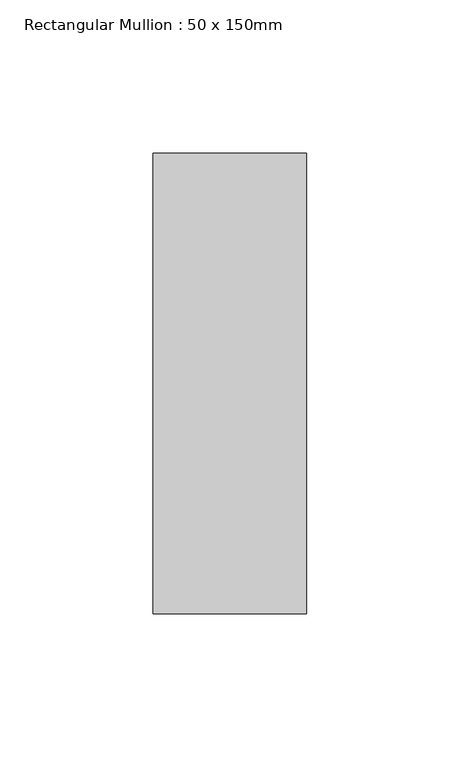
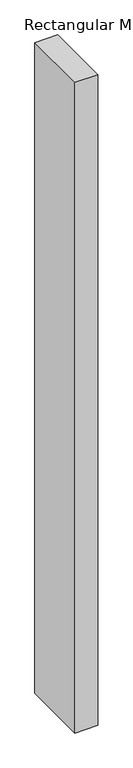
"""IFC4 building model written with IfcOpenShell, lengths in millimetres: member geometry, Rectangular Mullion : 50 x 150mm."""

from ifc_helpers import new_model, si_unit, frame, origin, place, context, project, spatial, polyline, outline, extrude, source, transform, mapped, element, save


def rectangular_mullion_50_x_150mm_7b69be1d(model_context):
    return source(origin(), model_context, "Body", "SweptSolid", [
        extrude(outline(polyline([(0.0, 75.0), (0.0, -75.0), (-50.0, -75.0), (-50.0, 75.0), (0.0, 75.0)])), frame((0.0, 0.0, -1490.0), z_axis=(0.0, 0.0, 1.0), x_axis=(1.0, 0.0, 0.0)), (0.0, 0.0, 1.0), 1490.0),
    ])


if __name__ == "__main__":
    model = new_model("IFC4")
    model_context = context("Model", 3, world=origin())
    ifc_project = project(units=[si_unit("LENGTHUNIT", "METRE", prefix="MILLI")], contexts=[model_context])
    site = spatial("IfcSite", under=ifc_project)
    building = spatial("IfcBuilding", under=site)
    placement = place(None, origin())
    rectangular_mullion_50_x_150mm_shape = rectangular_mullion_50_x_150mm_7b69be1d(model_context)
    element("IfcMember", 1, ObjectType="Rectangular Mullion : 50 x 150mm", at=placement, inside=building, context=model_context, shape_type="MappedRepresentation", body=[
        mapped(rectangular_mullion_50_x_150mm_shape, transform((0.0, 0.0, 0.0), x_axis=(1.0, 0.0, 0.0), y_axis=(0.0, 1.0, 0.0), z_axis=(0.0, 0.0, 1.0))),
    ])
    save(model, "model.ifc")

# Revit data of these elements
# Type "Rectangular Mullion : 50 x 150mm"
#   built-in parameter 1007304 = 0.492126 (stored number, unit not read)
#   built-in parameter 1007301 = 0.082021 (stored number, unit not read)
#   built-in parameter 1007300 = 0.082021 (stored number, unit not read)
# Element 1 (IfcMember, "Rectangular Mullion : 50 x 150mm")
#   Materials on its faces: "Aluminium"
# Materials
#   "Aluminium": class "Metal", colour RGB 247 247 247, transparency 0, Description = "Aluminium 6061", Cost = 0
